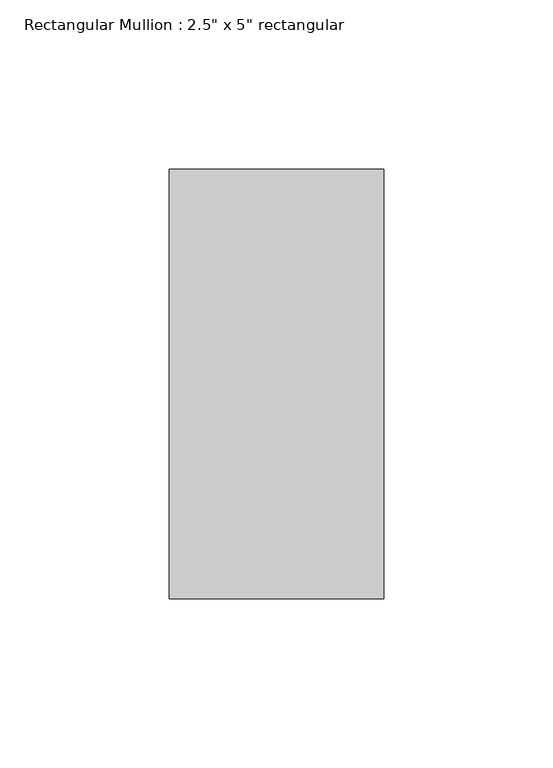
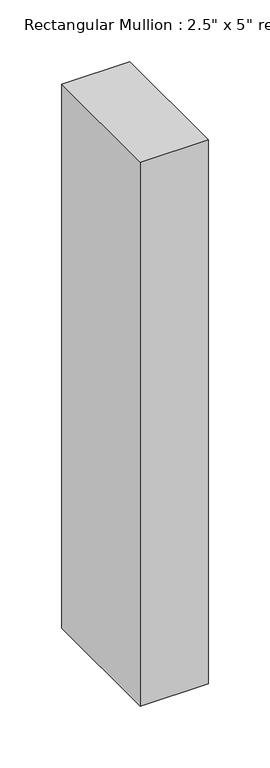
"""IFC4 building model written with IfcOpenShell, lengths in millimetres: member geometry."""

from ifc_helpers import new_model, si_unit, frame, origin, place, context, project, spatial, polyline, outline, extrude, source, transform, mapped, element, save


def member_3ed29256(model_context):
    return source(origin(), model_context, "Body", "SweptSolid", [
        extrude(outline(polyline([(0.0, 63.5), (0.0, -63.5), (-63.5, -63.5), (-63.5, 63.5), (0.0, 63.5)])), frame((0.0, 0.0, -537.6333333), z_axis=(0.0, 0.0, 1.0), x_axis=(1.0, 0.0, 0.0)), (0.0, 0.0, 1.0), 537.6333333),
    ])


if __name__ == "__main__":
    model = new_model("IFC4")
    model_context = context("Model", 3, world=origin())
    ifc_project = project(units=[si_unit("LENGTHUNIT", "METRE", prefix="MILLI")], contexts=[model_context])
    site = spatial("IfcSite", under=ifc_project)
    building = spatial("IfcBuilding", under=site)
    placement = place(None, origin())
    member_shape = member_3ed29256(model_context)
    element("IfcMember", 1, ObjectType="Rectangular Mullion : 2.5\" x 5\" rectangular", at=placement, inside=building, context=model_context, shape_type="MappedRepresentation", body=[
        mapped(member_shape, transform((0.0, 0.0, 0.0), x_axis=(1.0, 0.0, 0.0), y_axis=(0.0, 1.0, 0.0), z_axis=(0.0, 0.0, 1.0))),
    ])
    save(model, "model.ifc")

# Revit data of these elements
# Type "Rectangular Mullion : 2.5\" x 5\" rectangular"
#   built-in parameter 1007304 = 0.416667 (stored number, unit not read)
#   built-in parameter 1007301 = 0.104167 (stored number, unit not read)
#   built-in parameter 1007300 = 0.104167 (stored number, unit not read)
# Element 1 (IfcMember, "Rectangular Mullion : 2.5\" x 5\" rectangular")
#   Materials on its faces: "Aluminum"
# Materials
#   "Aluminum": class "Metal", colour RGB 247 247 247, transparency 0, Description = "Aluminum 6061", Cost = 0
